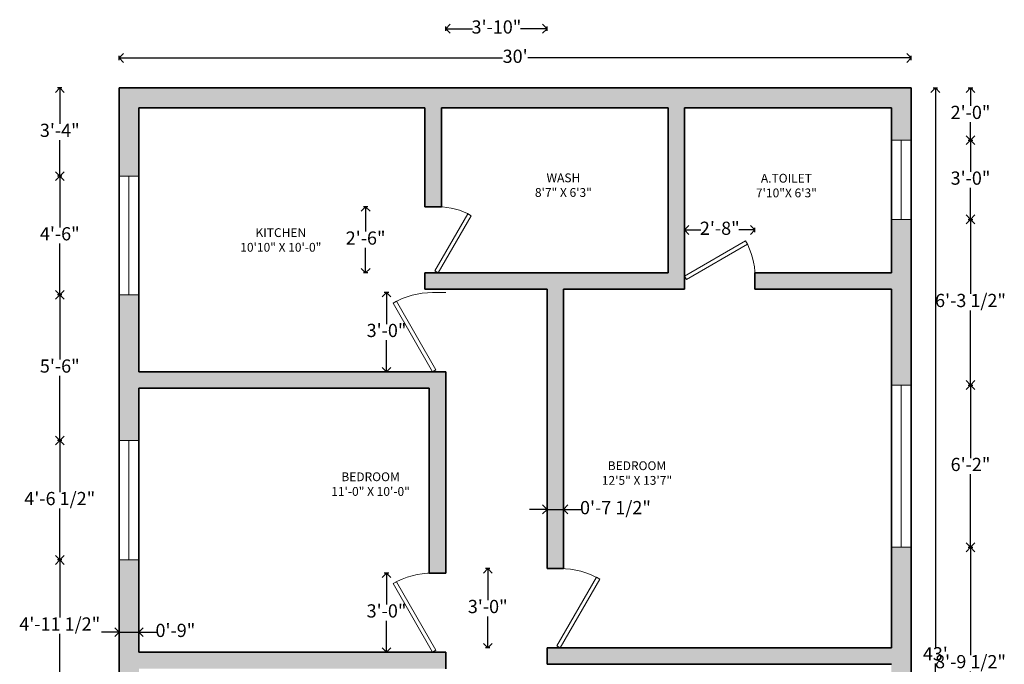
# Model space of a CAD drawing. Units: inches. Extents: x 2542 to 2989, y 529 to 1112.
# Tile 2 of 2: x 2542 to 2989, y 819 to 1112. Entities that reach past the tile are written whole.
import ezdxf

# ---------------------------------------------------------------- set-up
doc = ezdxf.new("R2010")
doc.units = ezdxf.units.IN
for name, color, linetype, lineweight in [('A-ANNO-DIMS', 2, 'Continuous', 18), ('A-AREA-IDEN', 7, 'Continuous', 18), ('A-DOOR', 3, 'Continuous', 18), ('A-GLAZ', 4, 'Continuous', 18), ('A-WALL', 7, 'Continuous', 35)]:
    doc.layers.add(name, color=color, linetype=linetype, lineweight=lineweight)
doc.layers.add('A-WALL-PATT', color=30, linetype='Continuous', lineweight=13, true_color=0xf26722)
doc.styles.get("Standard").update_dxf_attribs({"font": 'arial.ttf'})
doc.dimstyles.new('ISO-25', dxfattribs={"dimtxt": 6, "dimasz": 4, "dimexe": 1, "dimexo": 1, "dimtad": 0, "dimtih": 1, "dimtoh": 1, "dimlunit": 3, "dimtxsty": 'Standard', "dimblk": 'OPEN90', "dimcen": 2.5, "dimadec": 0, "dimazin": 0, "dimtfac": 1, "dimtmove": 0, "dimatfit": 3, "dimfxl": 1, "dimfxlon": 1, "dimarcsym": 0})

# ---------------------------------------------------------------- blocks, each defined once
blk = doc.blocks.new('*U11')
for p, q in [((0, 0), (0, -6)), ((36, 0), (36, -6))]:
    blk.add_line(p, q)
blk.add_lwpolyline([(0, 0), (31.18, 18), (32.05, 16.48), (0.87, -1.52)], close=True)
blk.add_arc((0, 0), 36, 0, 30)
blk = doc.blocks.new('*U5')
for p, q in [((0, 0), (0, 6)), ((36, 0), (36, 6))]:
    blk.add_line(p, q)
blk.add_lwpolyline([(0, 0), (31.18, -18), (32.05, -16.48), (0.88, 1.52)], close=True)
blk.add_arc((0, 0), 36, 330, 0)
blk = doc.blocks.new('*U3')
for p, q in [((0, 0), (0, -6)), ((32, 0), (32, -6))]:
    blk.add_line(p, q)
blk.add_lwpolyline([(0, 0), (27.71, 16), (28.59, 14.48), (0.87, -1.52)], close=True)
blk.add_arc((0, 0), 32, 0, 30)
blk = doc.blocks.new('*U10')
for p, q in [((0, 0), (0, 6)), ((36, 0), (36, 6))]:
    blk.add_line(p, q)
blk.add_lwpolyline([(0, 0), (31.18, -18), (32.05, -16.48), (0.87, 1.52)], close=True)
blk.add_arc((0, 0), 36, 330, 0)
blk = doc.blocks.new('*U7')
for p, q in [((0, 0), (0, 6)), ((30, 0), (30, 6))]:
    blk.add_line(p, q)
blk.add_lwpolyline([(0, 0), (25.98, -15), (26.86, -13.48), (0.87, 1.52)], close=True)
blk.add_arc((0, 0), 30, 330, 0)
blk = doc.blocks.new('_Open90')
at = {"color": 0, "linetype": 'ByBlock', "lineweight": -2}
for p, q in [((0, 0), (-1, 0)), ((-0.5, 0.5), (0, 0)), ((0, 0), (-0.5, -0.5))]:
    blk.add_line(p, q, dxfattribs=at)
blk = doc.blocks.new('*D12')
at = {"layer": 'A-ANNO-DIMS', "color": 0, "lineweight": -2, "transparency": 16777216}
for p, q in [((2587.06, 1093.63), (2587.06, 1095.63)), ((2591.06, 1094.63), (2761.35, 1094.63)), ((2943.06, 1094.63), (2772.77, 1094.63)), ((2947.06, 1093.63), (2947.06, 1095.63))]:
    blk.add_line(p, q, dxfattribs=at)
at = {"layer": 'Defpoints', "color": 0, "transparency": 16777216}
for p in [(2947.06, 1094.63), (2587.06, 1081), (2947.06, 1081)]:
    blk.add_point(p, dxfattribs=at)
at = {"layer": 'A-ANNO-DIMS', "color": 0, "lineweight": -2, "transparency": 16777216, "xscale": 4, "yscale": 4, "zscale": 4, "rotation": 180}
blk.add_blockref('_Open90', (2587.06, 1094.63), dxfattribs=at)
at = {"layer": 'A-ANNO-DIMS', "color": 0, "lineweight": -2, "transparency": 16777216, "xscale": 4, "yscale": 4, "zscale": 4}
blk.add_blockref('_Open90', (2947.06, 1094.63), dxfattribs=at)
at = {"layer": 'A-ANNO-DIMS', "color": 0, "transparency": 16777216, "insert": (2767.06, 1094.63), "char_height": 6, "attachment_point": 5}
blk.add_mtext("30'", dxfattribs=at)
blk = doc.blocks.new('*D13')
at = {"layer": 'A-ANNO-DIMS', "color": 0, "lineweight": -2, "transparency": 16777216}
for p, q in [((2957.03, 1081), (2959.03, 1081)), ((2958.03, 1077), (2958.03, 826.69)), ((2958.03, 569), (2958.03, 819.31)), ((2957.03, 565), (2959.03, 565))]:
    blk.add_line(p, q, dxfattribs=at)
at = {"layer": 'Defpoints', "color": 0, "transparency": 16777216}
for p in [(2947.06, 1081), (2947.06, 565), (2958.03, 565)]:
    blk.add_point(p, dxfattribs=at)
at = {"layer": 'A-ANNO-DIMS', "color": 0, "lineweight": -2, "transparency": 16777216, "xscale": 4, "yscale": 4, "zscale": 4}
for p, rotation in [((2958.03, 1081), 90), ((2958.03, 565), 270)]:
    blk.add_blockref('_Open90', p, dxfattribs=dict(at, rotation=rotation))
at = {"layer": 'A-ANNO-DIMS', "color": 0, "transparency": 16777216, "insert": (2958.03, 823), "char_height": 6, "attachment_point": 5}
blk.add_mtext("43'", dxfattribs=at)
blk = doc.blocks.new('*D18')
at = {"layer": 'A-ANNO-DIMS', "color": 0, "lineweight": -2, "transparency": 16777216}
for p, q in [((2561.11, 866.43), (2559.11, 866.43)), ((2560.11, 862.43), (2560.11, 840.29)), ((2560.11, 810.69), (2560.11, 832.83)), ((2561.11, 806.69), (2559.11, 806.69))]:
    blk.add_line(p, q, dxfattribs=at)
at = {"layer": 'Defpoints', "color": 0, "transparency": 16777216}
for p in [(2560.11, 866.43), (2587.06, 866.43), (2587.06, 806.69)]:
    blk.add_point(p, dxfattribs=at)
at = {"layer": 'A-ANNO-DIMS', "color": 0, "lineweight": -2, "transparency": 16777216, "xscale": 4, "yscale": 4, "zscale": 4}
for p, rotation in [((2560.11, 866.43), 90), ((2560.11, 806.69), 270)]:
    blk.add_blockref('_Open90', p, dxfattribs=dict(at, rotation=rotation))
at = {"layer": 'A-ANNO-DIMS', "color": 0, "transparency": 16777216, "insert": (2560.11, 836.56), "char_height": 6, "attachment_point": 5}
blk.add_mtext('4\'-11 1/2"', dxfattribs=at)
blk = doc.blocks.new('*D19')
at = {"layer": 'A-ANNO-DIMS', "color": 0, "lineweight": -2, "transparency": 16777216}
for p, q in [((2561.11, 920.71), (2559.11, 920.71)), ((2560.11, 916.71), (2560.11, 897.3)), ((2560.11, 870.43), (2560.11, 889.84)), ((2561.11, 866.43), (2559.11, 866.43))]:
    blk.add_line(p, q, dxfattribs=at)
at = {"layer": 'Defpoints', "color": 0, "transparency": 16777216}
for p in [(2560.11, 920.71), (2587.06, 920.71), (2587.06, 866.43)]:
    blk.add_point(p, dxfattribs=at)
at = {"layer": 'A-ANNO-DIMS', "color": 0, "lineweight": -2, "transparency": 16777216, "xscale": 4, "yscale": 4, "zscale": 4}
for p, rotation in [((2560.11, 920.71), 90), ((2560.11, 866.43), 270)]:
    blk.add_blockref('_Open90', p, dxfattribs=dict(at, rotation=rotation))
at = {"layer": 'A-ANNO-DIMS', "color": 0, "transparency": 16777216, "insert": (2560.11, 893.57), "char_height": 6, "attachment_point": 5}
blk.add_mtext('4\'-6 1/2"', dxfattribs=at)
blk = doc.blocks.new('*D20')
at = {"layer": 'A-ANNO-DIMS', "color": 0, "lineweight": -2, "transparency": 16777216}
for p, q in [((2561.11, 986.94), (2559.11, 986.94)), ((2560.11, 982.94), (2560.11, 957.51)), ((2560.11, 924.71), (2560.11, 950.13)), ((2561.11, 920.71), (2559.11, 920.71))]:
    blk.add_line(p, q, dxfattribs=at)
at = {"layer": 'Defpoints', "color": 0, "transparency": 16777216}
for p in [(2560.11, 986.94), (2587.06, 986.94), (2587.06, 920.71)]:
    blk.add_point(p, dxfattribs=at)
at = {"layer": 'A-ANNO-DIMS', "color": 0, "lineweight": -2, "transparency": 16777216, "xscale": 4, "yscale": 4, "zscale": 4}
for p, rotation in [((2560.11, 986.94), 90), ((2560.11, 920.71), 270)]:
    blk.add_blockref('_Open90', p, dxfattribs=dict(at, rotation=rotation))
at = {"layer": 'A-ANNO-DIMS', "color": 0, "transparency": 16777216, "insert": (2560.11, 953.82), "char_height": 6, "attachment_point": 5}
blk.add_mtext('5\'-6"', dxfattribs=at)
blk = doc.blocks.new('*D21')
at = {"layer": 'A-ANNO-DIMS', "color": 0, "lineweight": -2, "transparency": 16777216}
for p, q in [((2561.11, 1040.94), (2559.11, 1040.94)), ((2560.11, 1036.94), (2560.11, 1017.63)), ((2560.11, 990.94), (2560.11, 1010.25)), ((2561.11, 986.94), (2559.11, 986.94))]:
    blk.add_line(p, q, dxfattribs=at)
at = {"layer": 'Defpoints', "color": 0, "transparency": 16777216}
for p in [(2560.11, 1040.94), (2587.06, 1040.94), (2587.06, 986.94)]:
    blk.add_point(p, dxfattribs=at)
at = {"layer": 'A-ANNO-DIMS', "color": 0, "lineweight": -2, "transparency": 16777216, "xscale": 4, "yscale": 4, "zscale": 4}
for p, rotation in [((2560.11, 1040.94), 90), ((2560.11, 986.94), 270)]:
    blk.add_blockref('_Open90', p, dxfattribs=dict(at, rotation=rotation))
at = {"layer": 'A-ANNO-DIMS', "color": 0, "transparency": 16777216, "insert": (2560.11, 1013.94), "char_height": 6, "attachment_point": 5}
blk.add_mtext('4\'-6"', dxfattribs=at)
blk = doc.blocks.new('*D22')
at = {"layer": 'A-ANNO-DIMS', "color": 0, "lineweight": -2, "transparency": 16777216}
for p, q in [((2561.11, 1081), (2559.11, 1081)), ((2560.11, 1077), (2560.11, 1064.66)), ((2560.11, 1044.94), (2560.11, 1057.28)), ((2561.11, 1040.94), (2559.11, 1040.94))]:
    blk.add_line(p, q, dxfattribs=at)
at = {"layer": 'Defpoints', "color": 0, "transparency": 16777216}
for p in [(2560.11, 1081), (2587.06, 1081), (2587.06, 1040.94)]:
    blk.add_point(p, dxfattribs=at)
at = {"layer": 'A-ANNO-DIMS', "color": 0, "lineweight": -2, "transparency": 16777216, "xscale": 4, "yscale": 4, "zscale": 4}
for p, rotation in [((2560.11, 1081), 90), ((2560.11, 1040.94), 270)]:
    blk.add_blockref('_Open90', p, dxfattribs=dict(at, rotation=rotation))
at = {"layer": 'A-ANNO-DIMS', "color": 0, "transparency": 16777216, "insert": (2560.11, 1060.97), "char_height": 6, "attachment_point": 5}
blk.add_mtext('3\'-4"', dxfattribs=at)
blk = doc.blocks.new('*D25')
at = {"layer": 'A-ANNO-DIMS', "color": 0, "lineweight": -2, "transparency": 16777216}
for p, q in [((2973.01, 872.19), (2975.01, 872.19)), ((2974.01, 868.19), (2974.01, 823.16)), ((2974.01, 770.68), (2974.01, 815.71)), ((2973.01, 766.68), (2975.01, 766.68))]:
    blk.add_line(p, q, dxfattribs=at)
at = {"layer": 'Defpoints', "color": 0, "transparency": 16777216}
for p in [(2947.06, 872.19), (2974.01, 872.19), (2947.06, 766.68)]:
    blk.add_point(p, dxfattribs=at)
at = {"layer": 'A-ANNO-DIMS', "color": 0, "lineweight": -2, "transparency": 16777216, "xscale": 4, "yscale": 4, "zscale": 4}
for p, rotation in [((2974.01, 872.19), 90), ((2974.01, 766.68), 270)]:
    blk.add_blockref('_Open90', p, dxfattribs=dict(at, rotation=rotation))
at = {"layer": 'A-ANNO-DIMS', "color": 0, "transparency": 16777216, "insert": (2974.01, 819.43), "char_height": 6, "attachment_point": 5}
blk.add_mtext('8\'-9 1/2"', dxfattribs=at)
blk = doc.blocks.new('*D26')
at = {"layer": 'A-ANNO-DIMS', "color": 0, "lineweight": -2, "transparency": 16777216}
for p, q in [((2973.01, 945.97), (2975.01, 945.97)), ((2974.01, 941.97), (2974.01, 912.77)), ((2974.01, 876.19), (2974.01, 905.39)), ((2973.01, 872.19), (2975.01, 872.19))]:
    blk.add_line(p, q, dxfattribs=at)
at = {"layer": 'Defpoints', "color": 0, "transparency": 16777216}
for p in [(2947.06, 945.97), (2974.01, 945.97), (2947.06, 872.19)]:
    blk.add_point(p, dxfattribs=at)
at = {"layer": 'A-ANNO-DIMS', "color": 0, "lineweight": -2, "transparency": 16777216, "xscale": 4, "yscale": 4, "zscale": 4}
for p, rotation in [((2974.01, 945.97), 90), ((2974.01, 872.19), 270)]:
    blk.add_blockref('_Open90', p, dxfattribs=dict(at, rotation=rotation))
at = {"layer": 'A-ANNO-DIMS', "color": 0, "transparency": 16777216, "insert": (2974.01, 909.08), "char_height": 6, "attachment_point": 5}
blk.add_mtext('6\'-2"', dxfattribs=at)
blk = doc.blocks.new('*D27')
at = {"layer": 'A-ANNO-DIMS', "color": 0, "lineweight": -2, "transparency": 16777216}
for p, q in [((2973.01, 1021.27), (2975.01, 1021.27)), ((2974.01, 1017.27), (2974.01, 987.35)), ((2974.01, 949.97), (2974.01, 979.89)), ((2973.01, 945.97), (2975.01, 945.97))]:
    blk.add_line(p, q, dxfattribs=at)
at = {"layer": 'Defpoints', "color": 0, "transparency": 16777216}
for p in [(2947.06, 1021.27), (2974.01, 1021.27), (2947.06, 945.97)]:
    blk.add_point(p, dxfattribs=at)
at = {"layer": 'A-ANNO-DIMS', "color": 0, "lineweight": -2, "transparency": 16777216, "xscale": 4, "yscale": 4, "zscale": 4}
for p, rotation in [((2974.01, 1021.27), 90), ((2974.01, 945.97), 270)]:
    blk.add_blockref('_Open90', p, dxfattribs=dict(at, rotation=rotation))
at = {"layer": 'A-ANNO-DIMS', "color": 0, "transparency": 16777216, "insert": (2974.01, 983.62), "char_height": 6, "attachment_point": 5}
blk.add_mtext('6\'-3 1/2"', dxfattribs=at)
blk = doc.blocks.new('*D28')
at = {"layer": 'A-ANNO-DIMS', "color": 0, "lineweight": -2, "transparency": 16777216}
for p, q in [((2973.01, 1057.23), (2975.01, 1057.23)), ((2974.01, 1053.23), (2974.01, 1042.94)), ((2974.01, 1025.27), (2974.01, 1035.56)), ((2973.01, 1021.27), (2975.01, 1021.27))]:
    blk.add_line(p, q, dxfattribs=at)
at = {"layer": 'Defpoints', "color": 0, "transparency": 16777216}
for p in [(2947.06, 1057.23), (2974.01, 1057.23), (2947.06, 1021.27)]:
    blk.add_point(p, dxfattribs=at)
at = {"layer": 'A-ANNO-DIMS', "color": 0, "lineweight": -2, "transparency": 16777216, "xscale": 4, "yscale": 4, "zscale": 4}
for p, rotation in [((2974.01, 1057.23), 90), ((2974.01, 1021.27), 270)]:
    blk.add_blockref('_Open90', p, dxfattribs=dict(at, rotation=rotation))
at = {"layer": 'A-ANNO-DIMS', "color": 0, "transparency": 16777216, "insert": (2974.01, 1039.25), "char_height": 6, "attachment_point": 5}
blk.add_mtext('3\'-0"', dxfattribs=at)
blk = doc.blocks.new('*D29')
at = {"layer": 'A-ANNO-DIMS', "color": 0, "lineweight": -2, "transparency": 16777216}
for p, q in [((2973.01, 1081), (2975.01, 1081)), ((2974.01, 1077), (2974.01, 1072.81)), ((2974.01, 1061.23), (2974.01, 1065.43)), ((2973.01, 1057.23), (2975.01, 1057.23))]:
    blk.add_line(p, q, dxfattribs=at)
at = {"layer": 'Defpoints', "color": 0, "transparency": 16777216}
for p in [(2947.06, 1081), (2974.01, 1081), (2947.06, 1057.23)]:
    blk.add_point(p, dxfattribs=at)
at = {"layer": 'A-ANNO-DIMS', "color": 0, "lineweight": -2, "transparency": 16777216, "xscale": 4, "yscale": 4, "zscale": 4}
for p, rotation in [((2974.01, 1081), 90), ((2974.01, 1057.23), 270)]:
    blk.add_blockref('_Open90', p, dxfattribs=dict(at, rotation=rotation))
at = {"layer": 'A-ANNO-DIMS', "color": 0, "transparency": 16777216, "insert": (2974.01, 1069.12), "char_height": 6, "attachment_point": 5}
blk.add_mtext('2\'-0"', dxfattribs=at)
blk = doc.blocks.new('*D36')
at = {"layer": 'A-ANNO-DIMS', "color": 0, "lineweight": -2, "transparency": 16777216}
for p, q in [((2735.56, 1106.95), (2735.56, 1108.95)), ((2739.56, 1107.95), (2747.63, 1107.95)), ((2777.56, 1107.95), (2769.49, 1107.95)), ((2781.56, 1106.95), (2781.56, 1108.95))]:
    blk.add_line(p, q, dxfattribs=at)
at = {"layer": 'Defpoints', "color": 0, "transparency": 16777216}
for p in [(2781.56, 1107.95), (2735.56, 860.5), (2781.56, 862.5)]:
    blk.add_point(p, dxfattribs=at)
at = {"layer": 'A-ANNO-DIMS', "color": 0, "lineweight": -2, "transparency": 16777216, "xscale": 4, "yscale": 4, "zscale": 4, "rotation": 180}
blk.add_blockref('_Open90', (2735.56, 1107.95), dxfattribs=at)
at = {"layer": 'A-ANNO-DIMS', "color": 0, "lineweight": -2, "transparency": 16777216, "xscale": 4, "yscale": 4, "zscale": 4}
blk.add_blockref('_Open90', (2781.56, 1107.95), dxfattribs=at)
at = {"layer": 'A-ANNO-DIMS', "color": 0, "transparency": 16777216, "insert": (2758.56, 1107.95), "char_height": 6, "attachment_point": 5}
blk.add_mtext('3\'-10"', dxfattribs=at)
blk = doc.blocks.new('*D37')
at = {"layer": 'A-ANNO-DIMS', "color": 0, "lineweight": -2, "transparency": 16777216}
for p, q in [((2583.06, 833.64), (2579.06, 833.64)), ((2587.06, 832.64), (2587.06, 834.64)), ((2587.06, 833.64), (2596.06, 833.64)), ((2596.06, 832.64), (2596.06, 834.64)), ((2600.06, 833.64), (2604.06, 833.64))]:
    blk.add_line(p, q, dxfattribs=at)
at = {"layer": 'Defpoints', "color": 0, "transparency": 16777216}
for p in [(2596.06, 833.64), (2587.06, 806.69), (2596.06, 806.69)]:
    blk.add_point(p, dxfattribs=at)
at = {"layer": 'A-ANNO-DIMS', "color": 0, "lineweight": -2, "transparency": 16777216, "xscale": 4, "yscale": 4, "zscale": 4}
blk.add_blockref('_Open90', (2587.06, 833.64), dxfattribs=at)
at = {"layer": 'A-ANNO-DIMS', "color": 0, "lineweight": -2, "transparency": 16777216, "xscale": 4, "yscale": 4, "zscale": 4, "rotation": 180}
blk.add_blockref('_Open90', (2596.06, 833.64), dxfattribs=at)
at = {"layer": 'A-ANNO-DIMS', "color": 0, "transparency": 16777216, "insert": (2612.66, 833.64), "char_height": 6, "attachment_point": 5}
blk.add_mtext('0\'-9"', dxfattribs=at)
blk = doc.blocks.new('*D38')
at = {"layer": 'A-ANNO-DIMS', "color": 0, "lineweight": -2, "transparency": 16777216}
for p, q in [((2777.56, 889.45), (2773.56, 889.45)), ((2781.56, 888.45), (2781.56, 890.45)), ((2781.56, 889.45), (2789.06, 889.45)), ((2789.06, 888.45), (2789.06, 890.45)), ((2793.06, 889.45), (2797.06, 889.45))]:
    blk.add_line(p, q, dxfattribs=at)
at = {"layer": 'Defpoints', "color": 0, "transparency": 16777216}
for p in [(2789.06, 889.45), (2781.56, 862.5), (2789.06, 862.5)]:
    blk.add_point(p, dxfattribs=at)
at = {"layer": 'A-ANNO-DIMS', "color": 0, "lineweight": -2, "transparency": 16777216, "xscale": 4, "yscale": 4, "zscale": 4}
blk.add_blockref('_Open90', (2781.56, 889.45), dxfattribs=at)
at = {"layer": 'A-ANNO-DIMS', "color": 0, "lineweight": -2, "transparency": 16777216, "xscale": 4, "yscale": 4, "zscale": 4, "rotation": 180}
blk.add_blockref('_Open90', (2789.06, 889.45), dxfattribs=at)
at = {"layer": 'A-ANNO-DIMS', "color": 0, "transparency": 16777216, "insert": (2812.65, 889.45), "char_height": 6, "attachment_point": 5}
blk.add_mtext('0\'-7 1/2"', dxfattribs=at)
blk = doc.blocks.new('*D40')
at = {"layer": 'A-ANNO-DIMS', "color": 0, "lineweight": -2, "transparency": 16777216}
for p, q in [((2755.61, 862.5), (2753.61, 862.5)), ((2754.61, 858.5), (2754.61, 848.19)), ((2754.61, 830.5), (2754.61, 840.81)), ((2755.61, 826.5), (2753.61, 826.5))]:
    blk.add_line(p, q, dxfattribs=at)
at = {"layer": 'Defpoints', "color": 0, "transparency": 16777216}
for p in [(2754.61, 862.5), (2781.56, 862.5), (2781.56, 826.5)]:
    blk.add_point(p, dxfattribs=at)
at = {"layer": 'A-ANNO-DIMS', "color": 0, "lineweight": -2, "transparency": 16777216, "xscale": 4, "yscale": 4, "zscale": 4}
for p, rotation in [((2754.61, 862.5), 90), ((2754.61, 826.5), 270)]:
    blk.add_blockref('_Open90', p, dxfattribs=dict(at, rotation=rotation))
at = {"layer": 'A-ANNO-DIMS', "color": 0, "transparency": 16777216, "insert": (2754.61, 844.5), "char_height": 6, "attachment_point": 5}
blk.add_mtext('3\'-0"', dxfattribs=at)
blk = doc.blocks.new('*D41')
at = {"layer": 'A-ANNO-DIMS', "color": 0, "lineweight": -2, "transparency": 16777216}
for p, q in [((2844.06, 1015.45), (2844.06, 1017.45)), ((2848.06, 1016.45), (2851.41, 1016.45)), ((2872.06, 1016.45), (2868.71, 1016.45)), ((2876.06, 1015.45), (2876.06, 1017.45))]:
    blk.add_line(p, q, dxfattribs=at)
at = {"layer": 'Defpoints', "color": 0, "transparency": 16777216}
for p in [(2876.06, 1016.45), (2844.06, 989.5), (2876.06, 989.5)]:
    blk.add_point(p, dxfattribs=at)
at = {"layer": 'A-ANNO-DIMS', "color": 0, "lineweight": -2, "transparency": 16777216, "xscale": 4, "yscale": 4, "zscale": 4, "rotation": 180}
blk.add_blockref('_Open90', (2844.06, 1016.45), dxfattribs=at)
at = {"layer": 'A-ANNO-DIMS', "color": 0, "lineweight": -2, "transparency": 16777216, "xscale": 4, "yscale": 4, "zscale": 4}
blk.add_blockref('_Open90', (2876.06, 1016.45), dxfattribs=at)
at = {"layer": 'A-ANNO-DIMS', "color": 0, "transparency": 16777216, "insert": (2860.06, 1016.45), "char_height": 6, "attachment_point": 5}
blk.add_mtext('2\'-8"', dxfattribs=at)
blk = doc.blocks.new('*D42')
at = {"layer": 'A-ANNO-DIMS', "color": 0, "lineweight": -2, "transparency": 16777216}
for p, q in [((2700.11, 1027), (2698.11, 1027)), ((2699.11, 1023), (2699.11, 1015.69)), ((2699.11, 1001), (2699.11, 1008.31)), ((2700.11, 997), (2698.11, 997))]:
    blk.add_line(p, q, dxfattribs=at)
at = {"layer": 'Defpoints', "color": 0, "transparency": 16777216}
for p in [(2699.11, 1027), (2726.06, 1027), (2726.06, 997)]:
    blk.add_point(p, dxfattribs=at)
at = {"layer": 'A-ANNO-DIMS', "color": 0, "lineweight": -2, "transparency": 16777216, "xscale": 4, "yscale": 4, "zscale": 4}
for p, rotation in [((2699.11, 1027), 90), ((2699.11, 997), 270)]:
    blk.add_blockref('_Open90', p, dxfattribs=dict(at, rotation=rotation))
at = {"layer": 'A-ANNO-DIMS', "color": 0, "transparency": 16777216, "insert": (2699.11, 1012), "char_height": 6, "attachment_point": 5}
blk.add_mtext('2\'-6"', dxfattribs=at)
blk = doc.blocks.new('*D49')
at = {"layer": 'A-ANNO-DIMS', "color": 0, "lineweight": -2, "transparency": 16777216}
for p, q in [((2709.61, 860.5), (2707.61, 860.5)), ((2708.61, 856.5), (2708.61, 846.19)), ((2708.61, 828.5), (2708.61, 838.81)), ((2709.61, 824.5), (2707.61, 824.5))]:
    blk.add_line(p, q, dxfattribs=at)
at = {"layer": 'Defpoints', "color": 0, "transparency": 16777216}
for p in [(2708.61, 860.5), (2735.56, 860.5), (2735.56, 824.5)]:
    blk.add_point(p, dxfattribs=at)
at = {"layer": 'A-ANNO-DIMS', "color": 0, "lineweight": -2, "transparency": 16777216, "xscale": 4, "yscale": 4, "zscale": 4}
for p, rotation in [((2708.61, 860.5), 90), ((2708.61, 824.5), 270)]:
    blk.add_blockref('_Open90', p, dxfattribs=dict(at, rotation=rotation))
at = {"layer": 'A-ANNO-DIMS', "color": 0, "transparency": 16777216, "insert": (2708.61, 842.5), "char_height": 6, "attachment_point": 5}
blk.add_mtext('3\'-0"', dxfattribs=at)
blk = doc.blocks.new('*D50')
at = {"layer": 'A-ANNO-DIMS', "color": 0, "lineweight": -2, "transparency": 16777216}
for p, q in [((2709.61, 988), (2707.61, 988)), ((2708.61, 984), (2708.61, 973.69)), ((2708.61, 956), (2708.61, 966.31)), ((2709.61, 952), (2707.61, 952))]:
    blk.add_line(p, q, dxfattribs=at)
at = {"layer": 'Defpoints', "color": 0, "transparency": 16777216}
for p in [(2708.61, 988), (2735.56, 988), (2735.56, 952)]:
    blk.add_point(p, dxfattribs=at)
at = {"layer": 'A-ANNO-DIMS', "color": 0, "lineweight": -2, "transparency": 16777216, "xscale": 4, "yscale": 4, "zscale": 4}
for p, rotation in [((2708.61, 988), 90), ((2708.61, 952), 270)]:
    blk.add_blockref('_Open90', p, dxfattribs=dict(at, rotation=rotation))
at = {"layer": 'A-ANNO-DIMS', "color": 0, "transparency": 16777216, "insert": (2708.61, 970), "char_height": 6, "attachment_point": 5}
blk.add_mtext('3\'-0"', dxfattribs=at)

msp = doc.modelspace()

# ---------------------------------------------------------------- hatches: boundary and pattern name
at = {"layer": 'A-WALL-PATT'}
h = msp.add_hatch(color=256, dxfattribs=at)
h.dxf.hatch_style = 1
h.paths.add_polyline_path([(2947.06, 1081.002), (2587.06, 1081.002), (2587.06, 1040.94), (2596.06, 1040.94), (2596.06, 1072.002), (2726.06, 1072.002), (2726.06, 1027.002), (2726.093, 1027.002), (2733.56, 1027.002), (2733.56, 1072.002), (2836.56, 1072.002), (2836.56, 997.002), (2732.067, 997.002), (2732.06, 996.988), (2726.06, 997.002), (2726.06, 989.502), (2781.56, 989.502), (2781.56, 862.502), (2787.56, 862.502), (2789.06, 862.502), (2789.06, 989.502), (2844.06, 989.502), (2844.06, 995.502), (2844.06, 1072.002), (2938.06, 1072.002), (2938.06, 1057.232), (2947.06, 1057.232)])
h.paths.add_polyline_path([(2596.06, 944.502), (2728.06, 944.502), (2728.06, 860.502), (2735.56, 860.502), (2735.56, 952.002), (2729.56, 952.002), (2596.06, 952.002), (2596.06, 986.938), (2587.06, 986.938), (2587.06, 920.709), (2596.06, 920.709)])
h.paths.add_polyline_path([(2735.56, 824.502), (2729.56, 824.502), (2596.06, 824.502), (2596.06, 866.432), (2587.06, 866.432), (2587.06, 806.686), (2596.06, 806.686), (2596.06, 817.002), (2735.56, 817.002)])
h.paths.add_polyline_path([(2596.06, 763.869), (2587.06, 763.869), (2587.06, 709.221), (2596.06, 709.221)], flags=17)
h.paths.add_polyline_path([(2596.06, 653.502), (2735.56, 653.502), (2735.56, 659.502), (2735.56, 781.002), (2729.56, 781.002), (2728.06, 781.002), (2728.06, 661.002), (2596.06, 661.002), (2596.06, 672.254), (2587.06, 672.254), (2587.06, 565.002), (2603.045, 565.002), (2603.045, 574.002), (2596.06, 574.002)])
h.paths.add_polyline_path([(2894.269, 574.002), (2878.06, 574.002), (2878.06, 653.502), (2908.06, 653.502), (2908.06, 661.002), (2844.316, 661.002), (2844.316, 653.502), (2870.56, 653.502), (2870.56, 574.002), (2644.56, 574.002), (2644.56, 623.502), (2640.06, 623.502), (2640.06, 574.002), (2625.996, 574.002), (2625.996, 565.002), (2894.269, 565.002)])
h.paths.add_polyline_path([(2947.06, 702.099), (2938.06, 702.099), (2938.06, 574.002), (2920.298, 574.002), (2920.298, 565.002), (2947.06, 565.002)])
h.paths.add_polyline_path([(2947.06, 1021.275), (2938.06, 1021.275), (2938.06, 997.002), (2876.06, 997.002), (2876.06, 989.502), (2938.06, 989.502), (2938.06, 945.972), (2947.06, 945.972)], flags=17)
h.paths.add_polyline_path([(2947.06, 872.193), (2938.06, 872.193), (2938.06, 826.502), (2781.56, 826.502), (2781.56, 819.002), (2938.06, 819.002), (2938.06, 766.676), (2947.06, 766.676)])

# ---------------------------------------------------------------- linework, layer by layer
at = {"layer": 'A-GLAZ'}
for p, q in [((2938.06, 1057.232), (2947.06, 1057.232)), ((2942.56, 1057.232), (2942.56, 1021.275)), ((2596.06, 1040.94), (2587.06, 1040.94)), ((2591.56, 1040.94), (2591.56, 986.938)), ((2938.06, 1021.275), (2947.06, 1021.275)), ((2596.06, 986.938), (2587.06, 986.938)), ((2938.06, 945.972), (2947.06, 945.972)), ((2942.56, 945.972), (2942.56, 872.193)), ((2596.06, 920.709), (2587.06, 920.709)), ((2591.56, 920.709), (2591.56, 866.432)), ((2947.06, 872.193), (2938.06, 872.193)), ((2596.06, 866.432), (2587.06, 866.432))]:
    msp.add_line(p, q, dxfattribs=at)
at = {"layer": 'A-WALL'}
for p, q in [((2947.06, 1081.002), (2587.06, 1081.002)), ((2587.06, 1081.002), (2587.06, 565.002)), ((2947.06, 565.002), (2947.06, 1081.002)), ((2596.06, 1072.002), (2596.06, 952.002)), ((2726.06, 1072.002), (2596.06, 1072.002)), ((2726.06, 1072.002), (2726.06, 1027.002)), ((2733.56, 1072.002), (2733.56, 1027.002)), ((2836.56, 1072.002), (2733.56, 1072.002)), ((2836.56, 1072.002), (2836.56, 997.002)), ((2938.06, 1072.002), (2844.06, 1072.002)), ((2844.06, 1072.002), (2844.06, 989.502)), ((2938.06, 997.002), (2938.06, 1072.002)), ((2726.06, 1027.002), (2733.56, 1027.002)), ((2836.56, 997.002), (2726.06, 997.002)), ((2726.06, 997.002), (2726.06, 989.502)), ((2938.06, 997.002), (2876.06, 997.002)), ((2876.06, 997.002), (2876.06, 989.502)), ((2781.56, 989.502), (2726.06, 989.502)), ((2781.56, 989.502), (2781.56, 862.502)), ((2844.06, 989.502), (2789.06, 989.502)), ((2789.06, 862.502), (2789.06, 989.502)), ((2938.06, 989.502), (2876.06, 989.502)), ((2938.06, 826.502), (2938.06, 989.502)), ((2735.56, 952.002), (2596.06, 952.002)), ((2735.56, 952.002), (2735.56, 860.502)), ((2596.06, 944.502), (2728.06, 944.502)), ((2596.06, 944.502), (2596.06, 824.502)), ((2728.06, 944.502), (2728.06, 860.502)), ((2728.06, 860.502), (2735.56, 860.502)), ((2789.06, 862.502), (2781.56, 862.502)), ((2596.06, 824.502), (2735.56, 824.502)), ((2735.56, 824.502), (2735.56, 817.002)), ((2938.06, 826.502), (2781.56, 826.502)), ((2781.56, 826.502), (2781.56, 819.002)), ((2938.06, 819.002), (2781.56, 819.002))]:
    msp.add_line(p, q, dxfattribs=at)

# ---------------------------------------------------------------- block references
at = {"layer": 'A-DOOR'}
for name, p, rotation in [('*U7', (2732.06, 996.988), 89.87360472352675), ('*U11', (2729.56, 952.002), 90), ('*U5', (2787.56, 826.502), 90)]:
    msp.add_blockref(name, p, dxfattribs=dict(at, rotation=rotation))
msp.add_blockref('*U3', (2844.06, 995.502), dxfattribs=at)
at = {"layer": 'A-DOOR', "xscale": -1, "rotation": 270}
msp.add_blockref('*U10', (2729.56, 824.502), dxfattribs=at)

# ---------------------------------------------------------------- texts
at = {"layer": 'A-AREA-IDEN', "char_height": 4, "attachment_point": 1}
for s, insert in [('\\pxqc;WASH \\P8\'7" X 6\'3"', (2754.783, 1042.155)), ('\\pxqc;A.TOILET\\P7\'10"X 6\'3"', (2856.134, 1041.961)), ('\\pxqc;KITCHEN\\P10\'10" X 10\'-0"', (2626.354, 1017.239)), ('\\pxqc;BEDROOM\\P12\'5" X 13\'7"', (2788.204, 911.282)), ('\\pxqc;BEDROOM\\P11\'-0" X 10\'-0"', (2667.137, 906.252))]:
    msp.add_mtext_dynamic_manual_height_columns(s, width=68.42278, gutter_width=12.5, heights=[0], dxfattribs=dict(at, insert=insert))

# ---------------------------------------------------------------- dimensions: what is measured, and where the dimension line sits
at = {"layer": 'A-ANNO-DIMS'}
for base, p1, p2, override, picture, middle in [((2781.56, 1107.952), (2735.56, 860.502), (2781.56, 862.502), {"dimdec": 1, "dimlfac": 1, "dimrnd": 0, "dimzin": 1, "dimdsep": 46, "dimlunit": 4, "dimfrac": 2}, '*D36', (2758.56, 1107.952)), ((2947.06, 1094.631), (2587.06, 1081.002), (2947.06, 1081.002), {"dimclrd": 0, "dimclre": 0, "dimclrt": 0}, '*D12', (2767.06, 1094.631)), ((2876.06, 1016.452), (2844.06, 989.502), (2876.06, 989.502), {"dimdec": 1, "dimlfac": 1, "dimrnd": 0, "dimzin": 1, "dimdsep": 46, "dimlunit": 4, "dimfrac": 2}, '*D41', (2860.06, 1016.452)), ((2789.06, 889.452), (2781.56, 862.502), (2789.06, 862.502), {"dimdec": 1, "dimlfac": 1, "dimrnd": 0, "dimzin": 1, "dimdsep": 46, "dimlunit": 4, "dimfrac": 2}, '*D38', (2812.65, 889.452)), ((2596.06, 833.636), (2587.06, 806.686), (2596.06, 806.686), {"dimdec": 1, "dimlfac": 1, "dimrnd": 0, "dimzin": 1, "dimdsep": 46, "dimlunit": 4, "dimfrac": 2}, '*D37', (2612.659, 833.636))]:
    dim = msp.add_linear_dim(base=base, p1=p1, p2=p2, dimstyle='ISO-25', override=override, dxfattribs=at)
    dim.commit()
    dim.dimension.update_dxf_attribs({"geometry": picture, "text_midpoint": middle})
for base, p1, p2, override, picture, middle in [((2560.11, 1081.002), (2587.06, 1040.94), (2587.06, 1081.002), {"dimdec": 1, "dimlfac": 1, "dimrnd": 0, "dimzin": 1, "dimdsep": 46, "dimlunit": 4, "dimfrac": 2}, '*D22', (2560.11, 1060.971)), ((2958.029, 565.002), (2947.06, 1081.002), (2947.06, 565.002), {"dimclrd": 0, "dimclre": 0, "dimclrt": 0}, '*D13', (2958.029, 823.002)), ((2974.01, 1081.002), (2947.06, 1057.232), (2947.06, 1081.002), {"dimdec": 1, "dimlfac": 1, "dimrnd": 0, "dimzin": 1, "dimdsep": 46, "dimlunit": 4, "dimfrac": 2}, '*D29', (2974.01, 1069.117)), ((2974.01, 1057.232), (2947.06, 1021.275), (2947.06, 1057.232), {"dimdec": 1, "dimlfac": 1, "dimrnd": 0, "dimzin": 1, "dimdsep": 46, "dimlunit": 4, "dimfrac": 2}, '*D28', (2974.01, 1039.254)), ((2560.11, 1040.94), (2587.06, 986.938), (2587.06, 1040.94), {"dimdec": 1, "dimlfac": 1, "dimrnd": 0, "dimzin": 1, "dimdsep": 46, "dimlunit": 4, "dimfrac": 2}, '*D21', (2560.11, 1013.939)), ((2699.11, 1027.002), (2726.06, 997.002), (2726.06, 1027.002), {"dimdec": 1, "dimlfac": 1, "dimrnd": 0, "dimzin": 1, "dimdsep": 46, "dimlunit": 4, "dimfrac": 2}, '*D42', (2699.11, 1012.002)), ((2974.01, 1021.275), (2947.06, 945.972), (2947.06, 1021.275), {"dimdec": 1, "dimlfac": 1, "dimrnd": 0, "dimzin": 1, "dimdsep": 46, "dimlunit": 4, "dimfrac": 2}, '*D27', (2974.01, 983.623)), ((2560.11, 986.938), (2587.06, 920.709), (2587.06, 986.938), {"dimdec": 1, "dimlfac": 1, "dimrnd": 0, "dimzin": 1, "dimdsep": 46, "dimlunit": 4, "dimfrac": 2}, '*D20', (2560.11, 953.823)), ((2708.61, 988.002), (2735.56, 952.002), (2735.56, 988.002), {"dimdec": 1, "dimlfac": 1, "dimrnd": 0, "dimzin": 1, "dimdsep": 46, "dimlunit": 4, "dimfrac": 2}, '*D50', (2708.61, 970.002)), ((2974.01, 945.972), (2947.06, 872.193), (2947.06, 945.972), {"dimdec": 1, "dimlfac": 1, "dimrnd": 0, "dimzin": 1, "dimdsep": 46, "dimlunit": 4, "dimfrac": 2}, '*D26', (2974.01, 909.083)), ((2560.11, 920.709), (2587.06, 866.432), (2587.06, 920.709), {"dimdec": 1, "dimlfac": 1, "dimrnd": 0, "dimzin": 1, "dimdsep": 46, "dimlunit": 4, "dimfrac": 2}, '*D19', (2560.11, 893.57)), ((2974.01, 872.193), (2947.06, 766.676), (2947.06, 872.193), {"dimdec": 1, "dimlfac": 1, "dimrnd": 0, "dimzin": 1, "dimdsep": 46, "dimlunit": 4, "dimfrac": 2}, '*D25', (2974.01, 819.435)), ((2560.11, 866.432), (2587.06, 806.686), (2587.06, 866.432), {"dimdec": 1, "dimlfac": 1, "dimrnd": 0, "dimzin": 1, "dimdsep": 46, "dimlunit": 4, "dimfrac": 2}, '*D18', (2560.11, 836.559)), ((2708.61, 860.502), (2735.56, 824.502), (2735.56, 860.502), {"dimdec": 1, "dimlfac": 1, "dimrnd": 0, "dimzin": 1, "dimdsep": 46, "dimlunit": 4, "dimfrac": 2}, '*D49', (2708.61, 842.502)), ((2754.61, 862.502), (2781.56, 826.502), (2781.56, 862.502), {"dimdec": 1, "dimlfac": 1, "dimrnd": 0, "dimzin": 1, "dimdsep": 46, "dimlunit": 4, "dimfrac": 2}, '*D40', (2754.61, 844.502))]:
    dim = msp.add_linear_dim(base=base, p1=p1, p2=p2, angle=90, dimstyle='ISO-25', override=override, dxfattribs=at)
    dim.commit()
    dim.dimension.update_dxf_attribs({"geometry": picture, "text_midpoint": middle})

doc.saveas('drawing.dxf')
